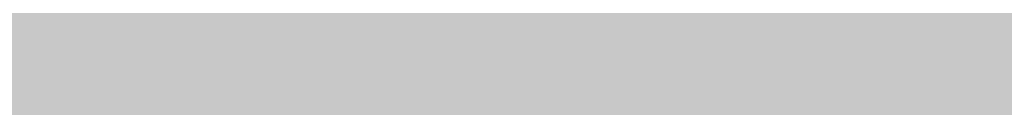
# Model space of a CAD drawing. Units: inches. Extents: x 2091 to 2899, y 967 to 2217.
# Tile 186 of 256: x 2203.16122 to 2203.18039, y 1152.24874 to 1152.25042. Entities that reach past the tile are written whole.
import ezdxf

# ---------------------------------------------------------------- set-up
doc = ezdxf.new("R2010")
doc.units = ezdxf.units.IN
doc.layers.add('A-WALL-PATT', color=141, linetype='Continuous', lineweight=13, true_color=0xadddf7)

msp = doc.modelspace()

# ---------------------------------------------------------------- hatches: boundary and pattern name
at = {"layer": 'A-WALL-PATT'}
h = msp.add_hatch(color=256, dxfattribs=at)
h.dxf.hatch_style = 1
h.paths.add_polyline_path([(2803.143603, 2050.919059), (2203.143603, 2050.919059), (2203.143603, 1090.919059), (2803.143603, 1090.919059)])
h.paths.add_polyline_path([(2635.79885, 1147.540465), (2674.524052, 1147.540465, 0.376086), (2678.529665, 1152.880202), (2678.529665, 1159.556473, 0.333335), (2674.524319, 1163.561846), (2674.524319, 1163.56185), (2674.524319, 1192.93439), (2635.805971, 1192.93439), (2597.087622, 1192.93439), (2597.087622, 1163.561846, 0.333335), (2593.082276, 1159.556473), (2593.082276, 1152.880202, 0.376086), (2597.087889, 1147.540465)], flags=0)
h.paths.add_polyline_path([(2436.010433, 1278.240778, 0.000483), (2435.952643, 1278.215027, -0.001328), (2435.935625, 1278.111693, -0.001711), (2436.11644, 1278.040758, 0.002185)], flags=0)
h.paths.add_polyline_path([(2794.143603, 1143.419059), (2794.143603, 1347.419059), (2543.370171, 1347.419059), (2543.370171, 1351.919059), (2794.143603, 1351.919059), (2794.143603, 1392.713555), (2793.947398, 1392.713555), (2793.947398, 1473.5369), (2794.143603, 1473.5369), (2794.143603, 1531.919059), (2650.143603, 1531.919059), (2650.143603, 1536.419059), (2794.143603, 1536.419059), (2794.143603, 1692.419059), (2609.375609, 1692.419059), (2609.375609, 1644.419059), (2604.875609, 1644.419059), (2604.875609, 1744.919059), (2609.375609, 1744.919059), (2609.375609, 1696.919059), (2794.143603, 1696.919059), (2794.143603, 1780.919059), (2609.643603, 1780.919059), (2493.875609, 1780.919059), (2493.875609, 1785.419059), (2609.643603, 1785.419059), (2794.143603, 1785.419059), (2794.143603, 1847.938821), (2793.951222, 1847.938821), (2793.951222, 1928.762166), (2794.143603, 1928.762166), (2794.143603, 1941.419059), (2614.143603, 1941.419059), (2614.143603, 1821.419059), (2609.643603, 1821.419059), (2609.643603, 1941.419059), (2392.143603, 1941.419059), (2392.143603, 1819.919059), (2387.643603, 1819.919059), (2387.643603, 1941.419059), (2212.143603, 1941.419059), (2212.143603, 1783.919059), (2392.143603, 1783.919059), (2392.143603, 1780.919059), (2212.143603, 1780.919059), (2212.143603, 1629.419059), (2387.643603, 1629.419059), (2387.643603, 1744.919059), (2392.143603, 1744.919059), (2392.143603, 1627.919059), (2317.143603, 1627.919059), (2317.143603, 1551.419059), (2317.143603, 1536.419059), (2459.383591, 1536.419059), (2459.383591, 1602.39648), (2463.883591, 1602.39648), (2463.883591, 1531.919059), (2456.643603, 1531.919059), (2456.643603, 1529.919059), (2452.143603, 1529.919059), (2452.143603, 1531.919059), (2312.643603, 1531.919059), (2312.643603, 1551.419059), (2306.143603, 1551.419059), (2306.143603, 1555.919059), (2308.143603, 1555.919059), (2308.143603, 1551.419059), (2312.643603, 1551.419059), (2312.643603, 1627.919059), (2212.143603, 1627.919059), (2212.143603, 1555.919059), (2270.143603, 1555.919059), (2270.143603, 1551.419059), (2212.143603, 1551.419059), (2212.143603, 1351.919059), (2272.143603, 1351.919059), (2272.143603, 1347.419059), (2212.143603, 1347.419059), (2212.143603, 1275.419059), (2308.143603, 1275.419059), (2308.143603, 1351.919059), (2452.143603, 1351.919059), (2452.143603, 1493.919059), (2456.643603, 1493.919059), (2456.643603, 1347.419059), (2312.643603, 1347.419059), (2312.643603, 1270.919059), (2212.143603, 1270.919059), (2212.143603, 1099.919059), (2281.237523, 1099.919059), (2282.871041, 1110.913803), (2282.008341, 1116.996603), (2278.557741, 1121.420403), (2268.205641, 1128.056203), (2272.087641, 1128.056203), (2273.812941, 1131.927003), (2279.420341, 1134.691903), (2285.027841, 1135.244903), (2287.615841, 1137.456803), (2288.047141, 1138.009803), (2289.341141, 1140.774703), (2291.066541, 1139.668703), (2292.360541, 1135.244903), (2295.379841, 1136.903803), (2296.242541, 1135.797903), (2297.105241, 1133.033003), (2300.124641, 1138.009803), (2303.143941, 1138.009803), (2304.437941, 1135.797903), (2303.143941, 1133.586003), (2306.594641, 1134.691903), (2307.888741, 1133.033003), (2310.908041, 1135.244903), (2313.927441, 1134.138903), (2315.62686, 1132.427102), (2308.320041, 1117.549603), (2290.203841, 1109.807903), (2288.909841, 1103.172103), (2289.272309, 1099.919059), (2434.918227, 1099.919059), (2431.593227, 1124.788059), (2429.930227, 1169.553059), (2430.927185, 1240.519694), (2435.658926, 1238.186126), (2437.135227, 1196.554059), (2438.798227, 1143.973059), (2442.678227, 1111.998059), (2446.558227, 1099.919059), (2794.143603, 1099.919059), (2794.143603, 1138.919059), (2548.032447, 1138.919059), (2548.032447, 1143.419059), (2548.032447, 1148.819059), (2546.668457, 1148.031559), (2528.685692, 1179.178622, 0.256256), (2512.032447, 1148.819059), (2512.032447, 1143.419059), (2512.032447, 1138.919059), (2507.532447, 1138.919059), (2507.532447, 1143.419059), (2507.532447, 1148.819059, 0.256256), (2490.879202, 1179.178622), (2472.896437, 1148.031559), (2471.532447, 1148.819059), (2471.532447, 1143.419059), (2467.032447, 1143.419059), (2467.032447, 1269.945786, 0.039061), (2460.909987, 1273.580059), (2467.032447, 1273.580059), (2467.032447, 1286.325364, 0.014511), (2465.216194, 1286.761905), (2467.032447, 1287.052576), (2467.032447, 1323.419059), (2471.532447, 1323.419059), (2471.532447, 1148.819059), (2489.532447, 1179.995973), (2490.896437, 1179.208473), (2490.879202, 1179.178622, -0.256256), (2507.532447, 1148.819059), (2507.532447, 1143.419059), (2512.032447, 1143.419059), (2512.032447, 1148.819059, -0.256256), (2528.685692, 1179.178622), (2528.668457, 1179.208473), (2530.032447, 1179.995973), (2548.032447, 1148.819059), (2548.032447, 1143.419059)], flags=16)
h.paths.add_polyline_path([(2607.768546, 1200.945083), (2607.768546, 1265.030625), (2597.087622, 1281.052011), (2619.784585, 1281.052011), (2627.795278, 1337.12686), (2635.79885, 1337.12686), (2643.816663, 1337.12686), (2651.827356, 1281.052011), (2674.524319, 1281.052011), (2663.843395, 1265.030625), (2663.843395, 1200.945083), (2635.805971, 1200.945083)], flags=0)
edge = h.paths.add_edge_path(flags=0)
edge.add_ellipse((13303.896215, 1272.998725), major_axis=(-10595.31304, 0.000001), ratio=0.842303870086, start_angle=0.6282372191, end_angle=0.6465540999, ccw=False)
edge.add_ellipse((2711.70045, 1156.852678), major_axis=(2.219769, 0), ratio=0.84230387, start_angle=111.535244, end_angle=180.628237, ccw=False)
edge.add_ellipse((13303.156292, 1272.998725), major_axis=(-10593.026306, 0), ratio=0.842303869544, start_angle=0.5282714718, end_angle=0.6465540971, ccw=False)
edge.add_line((2710.764596, 1175.333295), (2710.129986, 1175.333295))
edge.add_ellipse((2710.129986, 1176.579775), major_axis=(1.479846, 0), ratio=0.84230387, start_angle=180, end_angle=270, ccw=False)
edge.add_line((2708.65014, 1176.579775), (2708.65014, 1200.782914))
edge.add_ellipse((2710.129986, 1200.782914), major_axis=(1.479846, 0), ratio=0.84230387, start_angle=90, end_angle=180, ccw=False)
edge.add_line((2710.129986, 1202.029394), (2710.465075, 1202.029394))
edge.add_ellipse((13303.156292, 1272.998725), major_axis=(-10593.026306, 0), ratio=0.842303869544, start_angle=-0.0902290886, end_angle=0.3838667788, ccw=False)
edge.add_ellipse((2710.129986, 1290.927031), major_axis=(-1.479846, 0), ratio=0.84230387, start_angle=0, end_angle=90, ccw=False)
edge.add_line((2708.65014, 1290.927031), (2708.65014, 1315.13017))
edge.add_ellipse((2710.129986, 1315.13017), major_axis=(-1.479846, 0), ratio=0.84230387, start_angle=-90, end_angle=0, ccw=False)
edge.add_line((2710.129986, 1316.37665), (2710.706314, 1316.37665))
edge.add_ellipse((3238.40172, 1296.289566), major_axis=(528.234, 0), ratio=0.8423038695, start_angle=176.34957241, end_angle=177.82004969, ccw=False)
edge.add_ellipse((2775.063043, 1071.450696), major_axis=(313.307761, 0), ratio=0.8423038695, start_angle=102.12596555, end_angle=103.78052899, ccw=False)
edge.add_ellipse((2775.063043, 1078.305698), major_axis=(-305.302891, 0), ratio=0.8423038695, start_angle=-79.790461, end_angle=-77.55537271, ccw=False)
edge.add_ellipse((2695.141767, 1541.975383), major_axis=(-250.960216, 0), ratio=0.8423038695, start_angle=99.25656601, end_angle=102.55493264)
edge.add_line((2741.410326, 1334.214255), (2747.132545, 1337.378477))
edge.add_ellipse((2747.538616, 1336.857478), major_axis=(-0.739923, 0), ratio=0.8423039, start_angle=270, end_angle=307.93313, ccw=False)
edge.add_ellipse((2747.538616, 1336.857478), major_axis=(-0.739923, 0), ratio=0.8423039, start_angle=232.06687, end_angle=270, ccw=False)
edge.add_line((2747.944687, 1337.378477), (2753.666906, 1334.214255))
edge.add_ellipse((2799.935466, 1541.975383), major_axis=(250.960216, 0), ratio=0.8423038695, start_angle=257.44506736, end_angle=260.74343399)
edge.add_ellipse((2720.014189, 1078.305698), major_axis=(305.302891, 0), ratio=0.8423038695, start_angle=77.55537271, end_angle=79.790461, ccw=False)
edge.add_ellipse((2720.014189, 1071.450696), major_axis=(-313.307761, 0), ratio=0.8423038695, start_angle=256.21947101, end_angle=257.87403445, ccw=False)
edge.add_ellipse((2256.675512, 1296.289566), major_axis=(-528.234, 0), ratio=0.8423038695, start_angle=182.17995031, end_angle=183.65042759, ccw=False)
edge.add_line((2784.370918, 1316.37665), (2784.947247, 1316.37665))
edge.add_ellipse((2784.947247, 1315.13017), major_axis=(1.479846, 0), ratio=0.84230387, start_angle=0, end_angle=90, ccw=False)
edge.add_line((2786.427093, 1315.13017), (2786.427093, 1290.927031))
edge.add_ellipse((2784.947247, 1290.927031), major_axis=(1.479846, 0), ratio=0.84230387, start_angle=270, end_angle=360, ccw=False)
edge.add_ellipse((-7808.07906, 1272.998725), major_axis=(10593.026306, 0), ratio=0.842303869544, start_angle=-0.3838667788, end_angle=0.0902290886, ccw=False)
edge.add_line((2784.612157, 1202.029394), (2784.947247, 1202.029394))
edge.add_ellipse((2784.947247, 1200.782914), major_axis=(1.479846, 0), ratio=0.84230387, start_angle=0, end_angle=90, ccw=False)
edge.add_line((2786.427093, 1200.782914), (2786.427093, 1176.579775))
edge.add_ellipse((2784.947247, 1176.579775), major_axis=(-1.479846, 0), ratio=0.84230387, start_angle=90, end_angle=180, ccw=False)
edge.add_line((2784.947247, 1175.333295), (2784.312636, 1175.333295))
edge.add_ellipse((-7808.07906, 1272.998725), major_axis=(10593.026306, 0), ratio=0.842303869544, start_angle=-0.6186431963, end_angle=-0.5282714718, ccw=False)
edge.add_ellipse((2783.376783, 1156.852678), major_axis=(-2.219769, 0), ratio=0.84230387, start_angle=179.371763, end_angle=248.464757, ccw=False)
edge.add_ellipse((-7808.818983, 1272.998725), major_axis=(-10595.31304, 0.000004), ratio=0.842303865762, start_angle=179.3534459226, end_angle=179.3717628034, ccw=False)
edge.add_ellipse((2780.297303, 1153.500793), major_axis=(-5.246426, 0), ratio=0.84230387, start_angle=90, end_angle=179.353446, ccw=False)
edge.add_line((2780.297303, 1149.081708), (2714.77993, 1149.081708))
edge.add_ellipse((2714.77993, 1153.500793), major_axis=(5.246426, 0), ratio=0.84230387, start_angle=180.646554, end_angle=270, ccw=False)
edge = h.paths.add_edge_path(flags=0)
edge.add_line((2718.187367, 1151.007833), (2718.187367, 1170.472364))
edge.add_ellipse((2721.14706, 1170.472364), major_axis=(-2.959692, 0), ratio=0.84230387, start_angle=-90, end_angle=0, ccw=False)
edge.add_line((2721.14706, 1172.965324), (2773.930173, 1172.965324))
edge.add_ellipse((2773.930173, 1170.472364), major_axis=(-2.959692, 0), ratio=0.84230387, start_angle=180, end_angle=270, ccw=False)
edge.add_line((2776.889865, 1170.472364), (2776.889865, 1151.007833))
edge.add_line((2776.889865, 1151.007833), (2718.187367, 1151.007833))
edge = h.paths.add_edge_path(flags=0)
edge.add_line((2718.187367, 1180.23415), (2718.187367, 1199.057834))
edge.add_ellipse((2747.538616, 1320.39864), major_axis=(147.017924, 0), ratio=0.8423038695, start_angle=256.40186531, end_angle=283.59813469)
edge.add_line((2776.889865, 1199.057834), (2776.889865, 1180.23415))
edge.add_ellipse((2747.538616, 1301.574956), major_axis=(147.017924, 0), ratio=0.8423038695, start_angle=256.40186531, end_angle=283.59813469, ccw=False)
edge = h.paths.add_edge_path(flags=0)
edge.add_ellipse((13303.156292, 1272.998725), major_axis=(-10591.54646, 0), ratio=0.842303869555, start_angle=0.0555943135, end_angle=0.3777641939, ccw=False)
edge.add_line((2711.616859, 1262.72171), (2715.667408, 1249.495396))
edge.add_ellipse((6413.891963, 1241.691919), major_axis=(-3698.236159, 0), ratio=0.84230386955, start_angle=-0.120897369, end_angle=0.364076349)
edge.add_line((2715.761038, 1218.192455), (2711.934307, 1203.167361))
edge = h.paths.add_edge_path(flags=0)
edge.add_line((2718.187367, 1251.074566), (2716.002485, 1267.450435))
edge.add_ellipse((2742.151175, 1202.18954), major_axis=(81.772585, 0), ratio=0.84230387, start_angle=94.27742096, end_angle=111.8349538, ccw=False)
edge.add_line((2737.009748, 1270.930626), (2758.067484, 1270.930626))
edge.add_ellipse((2752.926058, 1202.18954), major_axis=(81.772585, 0), ratio=0.84230387, start_angle=68.1650462, end_angle=85.72257904, ccw=False)
edge.add_line((2779.074747, 1267.450435), (2776.889865, 1251.074566))
edge.add_ellipse((2750.338059, 1187.885356), major_axis=(79.579664, 0), ratio=0.84230387, start_angle=67.20808512, end_angle=85.1299304)
edge.add_line((2756.034656, 1254.743656), (2739.042576, 1254.743656))
edge.add_ellipse((2744.739174, 1187.885356), major_axis=(79.579664, 0), ratio=0.84230387, start_angle=94.8700696, end_angle=112.79191488)
edge = h.paths.add_edge_path(flags=0)
edge.add_line((2783.142926, 1203.167361), (2779.316194, 1218.192455))
edge.add_ellipse((-918.81473, 1241.691919), major_axis=(3698.236159, 0), ratio=0.84230386955, start_angle=-0.364076349, end_angle=0.120897369)
edge.add_line((2779.409825, 1249.495396), (2783.460373, 1262.72171))
edge.add_ellipse((-7808.07906, 1272.998725), major_axis=(-10591.54646, 0), ratio=0.84230386954, start_angle=179.6222358061, end_angle=179.9444056865, ccw=False)
edge = h.paths.add_edge_path(flags=0)
edge.add_ellipse((2734.200892, 1286.69044), major_axis=(-0.356609, 6.340078), ratio=0.60383358, start_angle=89.0020143, end_angle=253.657408, ccw=False)
edge.add_line((2730.369001, 1286.541806), (2730.369001, 1301.35198))
edge.add_line((2730.369001, 1301.35198), (2735.913311, 1305.214803))
edge.add_ellipse((2736.384917, 1304.734561), major_axis=(0.739923, 0), ratio=0.8423039, start_angle=90, end_angle=134.480211, ccw=False)
edge.add_line((2736.384917, 1305.357801), (2738.032783, 1305.357801))
edge.add_line((2738.032783, 1305.357801), (2738.032783, 1307.707927))
edge.add_ellipse((2794.201642, 1307.707927), major_axis=(56.168859, 0), ratio=0.84230387, start_angle=150.5614304, end_angle=180, ccw=False)
edge.add_ellipse((2700.875591, 1307.707927), major_axis=(-56.168859, 0), ratio=0.84230387, start_angle=180, end_angle=209.4385696, ccw=False)
edge.add_line((2757.04445, 1307.707927), (2757.04445, 1305.357801))
edge.add_line((2757.04445, 1305.357801), (2758.692316, 1305.357801))
edge.add_ellipse((2758.692316, 1304.734561), major_axis=(-0.739923, 0), ratio=0.8423039, start_angle=225.519789, end_angle=270, ccw=False)
edge.add_line((2759.163922, 1305.214803), (2764.708231, 1301.35198))
edge.add_line((2764.708231, 1301.35198), (2764.708231, 1286.541806))
edge.add_ellipse((2760.87634, 1286.69044), major_axis=(0.356609, 6.340078), ratio=0.60383358, start_angle=106.342592, end_angle=270.9979857, ccw=False)
edge.add_line((2757.04445, 1285.79709), (2757.04445, 1307.707927))
edge.add_ellipse((2700.875591, 1307.707927), major_axis=(-56.168859, 0), ratio=0.84230387, start_angle=180, end_angle=209.4385696)
edge.add_ellipse((2794.201642, 1307.707927), major_axis=(56.168859, 0), ratio=0.84230387, start_angle=150.5614304, end_angle=180)
edge.add_line((2738.032783, 1307.707927), (2738.032783, 1285.79709))
h.paths.add_polyline_path([(2417.812273, 1104.449704), (2413.492273, 1102.529704), (2410.612273, 1103.969704), (2409.172273, 1106.369704), (2407.252273, 1107.329704), (2406.292273, 1109.729704), (2405.332273, 1114.049704), (2405.332273, 1117.889704), (2406.292273, 1120.129704), (2407.252273, 1119.809704), (2408.848322, 1118.327658), (2410.173945, 1119.42417), (2410.211273, 1120.405704), (2411.040731, 1121.419054), (2410.699273, 1119.858704), (2410.173945, 1119.42417), (2410.088452, 1117.176109), (2411.132836, 1116.206324), (2413.972273, 1119.329704), (2416.852273, 1120.769704), (2416.869721, 1120.798784), (2417.035071, 1119.405116), (2417.896213, 1118.143384), (2418.292273, 1118.369704), (2419.544447, 1120.039269), (2419.360915, 1118.387487), (2419.032108, 1119.356151), (2418.398939, 1118.511926), (2419.252273, 1114.529704), (2418.794091, 1107.198795)], flags=0)
h.paths.add_polyline_path([(2508.870171, 1347.419059), (2508.370171, 1347.419059), (2508.370171, 1351.919059), (2508.870171, 1351.919059)], flags=0)
h.paths.add_polyline_path([(2473.370171, 1347.419059), (2472.370171, 1347.419059), (2467.870171, 1347.419059), (2467.870171, 1455.419059), (2472.370171, 1455.419059), (2472.370171, 1352.419059), (2473.370171, 1352.419059)], flags=0)
h.paths.add_polyline_path([(2352.106244, 1217.446197), (2349.226244, 1218.886197), (2347.786244, 1221.286197), (2345.866244, 1222.246197), (2344.906244, 1224.646197), (2343.946244, 1228.966197), (2343.946244, 1232.806197), (2344.906244, 1235.046197), (2345.866244, 1234.726197), (2347.462293, 1233.244152), (2348.787916, 1234.340663), (2348.825244, 1235.322197), (2349.654702, 1236.335547), (2349.313244, 1234.775197), (2348.787916, 1234.340663), (2348.702423, 1232.092603), (2349.746807, 1231.122817), (2352.586244, 1234.246197), (2355.466244, 1235.686197), (2355.483692, 1235.715277), (2355.649043, 1234.321609), (2356.510185, 1233.059877), (2356.906244, 1233.286197), (2358.158418, 1234.955762), (2357.974887, 1233.30398), (2357.646079, 1234.272644), (2357.012911, 1233.428419), (2357.866244, 1229.446197), (2357.408062, 1222.115288), (2356.426244, 1219.366197)], flags=0)
h.paths.add_polyline_path([(2348.2968, 1112.22442), (2347.0138, 1112.31042), (2345.5298, 1114.12742), (2345.7318, 1115.85842), (2346.8118, 1116.98242), (2346.8118, 1114.64642), (2345.8668, 1114.21442), (2346.8798, 1114.30042)], flags=0)
h.paths.add_polyline_path([(2347.0138, 1110.92642), (2346.2718, 1110.49342), (2346.6098, 1111.18642)], flags=0)
h.paths.add_polyline_path([(2345.8668, 1118.19442), (2345.5298, 1117.32942), (2343.7078, 1118.02142), (2344.3828, 1118.62642)], flags=0)
h.paths.add_polyline_path([(2346.6768, 1109.28242), (2346.0698, 1108.07142), (2345.8668, 1110.06142)], flags=0)
h.paths.add_polyline_path([(2345.0568, 1119.75142), (2343.6398, 1119.75142), (2343.9778, 1121.13542)], flags=0)
h.paths.add_polyline_path([(2345.2598, 1116.55042), (2345.1248, 1115.85842), (2344.9218, 1115.68542), (2344.7198, 1116.37742)], flags=0)
h.paths.add_polyline_path([(2345.6648, 1112.31042), (2345.4618, 1111.53242), (2344.0448, 1111.96442), (2344.6518, 1112.57042)], flags=0)
h.paths.add_polyline_path([(2345.1918, 1113.34942), (2344.4498, 1113.86842), (2344.7198, 1114.38742)], flags=0)
h.paths.add_polyline_path([(2344.6518, 1116.80942), (2344.1798, 1115.68542), (2344.6518, 1115.33942), (2343.9098, 1114.90642), (2343.0328, 1115.94442), (2343.6398, 1116.46342)], flags=0)
h.paths.add_polyline_path([(2345.8668, 1106.68642), (2344.9898, 1105.56242), (2344.5168, 1106.60042)], flags=0)
h.paths.add_polyline_path([(2344.8548, 1110.06142), (2344.5168, 1109.28242), (2344.1128, 1109.71542)], flags=0)
h.paths.add_polyline_path([(2344.0448, 1113.52242), (2343.4378, 1113.08942), (2342.7628, 1113.95442)], flags=0)
h.paths.add_polyline_path([(2344.3148, 1111.01242), (2342.9648, 1110.32042), (2342.9648, 1111.09942)], flags=0)
h.paths.add_polyline_path([(2345.1248, 1104.69742), (2344.5848, 1103.74542), (2344.4498, 1104.26442)], flags=0)
h.paths.add_polyline_path([(2342.8298, 1121.22242), (2341.7498, 1120.53042), (2340.5358, 1121.04942), (2340.1308, 1121.82842), (2340.6708, 1122.95242), (2341.1428, 1121.82842), (2341.6148, 1122.00142)], flags=0)
h.paths.add_polyline_path([(2342.9648, 1119.75142), (2343.0328, 1118.45342), (2342.0878, 1118.02142), (2342.0198, 1119.49142)], flags=0)
h.paths.add_polyline_path([(2342.6948, 1116.89642), (2341.9528, 1116.63642), (2342.0198, 1117.32942)], flags=0)
h.paths.add_polyline_path([(2343.0328, 1112.22442), (2342.0198, 1111.79142), (2341.5478, 1112.22442), (2342.3578, 1113.34942)], flags=0)
h.paths.add_polyline_path([(2343.7748, 1104.43742), (2342.6278, 1102.88042), (2342.6948, 1104.61042), (2343.4378, 1105.12942)], flags=0)
h.paths.add_polyline_path([(2342.0198, 1115.07942), (2340.8058, 1115.51242), (2340.9408, 1116.37742)], flags=0)
h.paths.add_polyline_path([(2341.4808, 1120.09742), (2341.4808, 1119.40542), (2341.0758, 1119.57842), (2341.1428, 1120.09742)], flags=0)
h.paths.add_polyline_path([(2341.8178, 1114.47342), (2340.9408, 1113.08942), (2340.8058, 1114.56042)], flags=0)
h.paths.add_polyline_path([(2341.1428, 1118.54042), (2340.9408, 1116.98242), (2339.0508, 1117.67542), (2339.0508, 1118.62642)], flags=0)
h.paths.add_polyline_path([(2342.6948, 1101.66842), (2341.9528, 1101.84142), (2342.5598, 1102.36142)], flags=0)
h.paths.add_polyline_path([(2340.3328, 1119.66542), (2338.4438, 1119.57842), (2337.9038, 1120.35742), (2339.6578, 1120.61642)], flags=0)
h.paths.add_polyline_path([(2340.3328, 1115.33942), (2340.0628, 1113.69542), (2339.3878, 1115.33942)], flags=0)
h.paths.add_polyline_path([(2341.8178, 1103.83142), (2341.5478, 1102.88042), (2341.1428, 1103.65842)], flags=0)
h.paths.add_polyline_path([(2339.0508, 1122.86642), (2337.2958, 1121.82842), (2337.0938, 1123.12542), (2337.7688, 1123.81842)], flags=0)
h.paths.add_polyline_path([(2339.1178, 1121.74142), (2338.8478, 1121.22242), (2338.1738, 1121.04942), (2338.3758, 1121.56842)], flags=0)
h.paths.add_polyline_path([(2339.1858, 1119.31942), (2338.6458, 1118.71342), (2338.2408, 1118.10742), (2338.2408, 1118.88642)], flags=0)
h.paths.add_polyline_path([(2341.1428, 1101.92842), (2340.6028, 1101.23642), (2340.0628, 1101.84142), (2340.6028, 1102.36142)], flags=0)
h.paths.add_polyline_path([(2337.6338, 1117.76142), (2336.6208, 1118.28042), (2337.2958, 1118.97242)], flags=0)
h.paths.add_polyline_path([(2336.8238, 1119.57842), (2334.7988, 1118.97242), (2335.2038, 1120.35742), (2336.5538, 1120.87642)], flags=0)
h.paths.add_polyline_path([(2339.1178, 1100.45742), (2337.3638, 1100.54342), (2336.7558, 1101.23642)], flags=0)
h.paths.add_polyline_path([(2336.3508, 1122.43342), (2336.0138, 1121.91442), (2334.9338, 1122.43342), (2334.5288, 1123.47142), (2335.7438, 1122.77942)], flags=0)
h.paths.add_polyline_path([(2334.7318, 1120.87642), (2334.2588, 1120.35742), (2334.0568, 1120.78942), (2334.5968, 1121.30842)], flags=0)
h.paths.add_polyline_path([(2334.4618, 1122.17442), (2332.5718, 1121.30842), (2331.3568, 1122.17442), (2332.0998, 1122.86642)], flags=0)
h.paths.add_polyline_path([(2334.2588, 1118.54042), (2333.3818, 1118.45342), (2333.6518, 1119.31942)], flags=0)
h.paths.add_polyline_path([(2335.5418, 1102.27442), (2334.1918, 1102.62042), (2335.2718, 1103.31242)], flags=0)
h.paths.add_polyline_path([(2332.7068, 1119.66542), (2331.6948, 1120.44342), (2332.5048, 1120.78942)], flags=0)
h.paths.add_polyline_path([(2334.7318, 1101.14942), (2333.5168, 1101.58242), (2333.9888, 1101.75542)], flags=0)
h.paths.add_polyline_path([(2332.6398, 1116.63642), (2331.0868, 1116.29042), (2331.9648, 1118.19442)], flags=0)
h.paths.add_polyline_path([(2330.7498, 1121.56842), (2330.2768, 1120.27042), (2328.5228, 1119.31942), (2328.9948, 1121.04942)], flags=0)
h.paths.add_polyline_path([(2330.7498, 1118.62642), (2330.0078, 1117.50242), (2329.8728, 1118.02142)], flags=0)
h.paths.add_polyline_path([(2332.0998, 1102.36142), (2330.5468, 1102.01442), (2331.6948, 1102.96642)], flags=0)
h.paths.add_polyline_path([(2329.5348, 1113.60842), (2329.0628, 1112.31042), (2328.5898, 1113.34942)], flags=0)
h.paths.add_polyline_path([(2328.3878, 1117.84842), (2327.5098, 1116.55042), (2327.1728, 1117.76142)], flags=0)
h.paths.add_polyline_path([(2329.7378, 1106.51342), (2329.5348, 1105.30242), (2328.2528, 1106.08142)], flags=0)
h.paths.add_polyline_path([(2328.6578, 1114.38742), (2328.0498, 1114.12742), (2328.3198, 1114.90642)], flags=0)
h.paths.add_polyline_path([(2328.3198, 1112.22442), (2327.1058, 1112.13742), (2326.7008, 1112.65642)], flags=0)
h.paths.add_polyline_path([(2326.9028, 1115.25242), (2326.7008, 1114.12742), (2325.2158, 1113.60842), (2326.0928, 1115.33942)], flags=0)
h.paths.add_polyline_path([(2326.6328, 1108.33042), (2326.0928, 1107.37942), (2325.8908, 1108.50342), (2326.4978, 1109.10942)], flags=0)
h.paths.add_polyline_path([(2615.143603, 1531.919059), (2609.643603, 1531.919059), (2609.643603, 1620.419059), (2614.143603, 1620.419059), (2614.143603, 1536.419059), (2615.143603, 1536.419059)], flags=0)
h.paths.add_polyline_path([(2545.143603, 1563.419059), (2464.143603, 1563.419059), (2464.143603, 1632.419059), (2509.143603, 1632.419059), (2509.143603, 1627.919059), (2509.143603, 1603.919059), (2468.643603, 1603.919059), (2468.643603, 1567.919059), (2540.643603, 1567.919059), (2540.643603, 1591.919059), (2545.143603, 1591.919059)], flags=0)
h.paths.add_polyline_path([(2388.969048, 1549.985735), (2357.434181, 1549.985735), (2357.434181, 1623.360778), (2399.362777, 1623.360778), (2435.689465, 1623.360778), (2435.592547, 1602.559273), (2435.592547, 1602.39648), (2388.969048, 1602.39648)], flags=0)
h.paths.add_polyline_path([(2388.880628, 1555.809151), (2374.904429, 1555.809151), (2374.904429, 1600.571564), (2374.904429, 1615.457645), (2406.350877, 1615.457645), (2406.350877, 1618.939431), (2412.174293, 1615.457645), (2406.350877, 1611.97586), (2406.350877, 1615.457645), (2388.880628, 1615.457645)], flags=0)
h.paths.add_polyline_path([(2568.875609, 1644.419059), (2453.375609, 1644.419059), (2453.375609, 1785.419059), (2457.875609, 1785.419059), (2457.875609, 1648.919059), (2568.875609, 1648.919059)], flags=0)
h.paths.add_polyline_path([(2212.143603, 1945.919059), (2212.143603, 2041.919059), (2794.143603, 2041.919059), (2794.143603, 1945.919059)], flags=16)
h.paths.add_polyline_path([(2271.082728, 1964.317238), (2776.852968, 1964.317238), (2776.852968, 2037.169623), (2271.082728, 2037.169623)], flags=8)
h.paths.add_polyline_path([(2380.649285, 1536.824144), (2461.040809, 1536.824144), (2461.040809, 1554.652587), (2380.649285, 1554.652587)], flags=8)
h.paths.add_polyline_path([(2240.755709, 1609.725451), (2309.185829, 1609.725451), (2309.185829, 1617.698204), (2240.755709, 1617.698204)], flags=8)
h.paths.add_polyline_path([(2212.677255, 1313.504102), (2282.59152, 1313.504102), (2282.59152, 1322.745239), (2212.677255, 1322.745239)], flags=8)
h.paths.add_polyline_path([(2457.111976, 1114.778574), (2558.481581, 1114.778574), (2558.481581, 1142.219682), (2457.111976, 1142.219682)], flags=8)
h.paths.add_polyline_path([(2473.442337, 1273.010067), (2604.641226, 1273.010067), (2604.641226, 1318.346935), (2473.442337, 1318.346935)], flags=8)
h.paths.add_polyline_path([(2638.876302, 1626.977432), (2684.250367, 1627.976738), (2684.038483, 1637.597494), (2638.664417, 1636.598188)], flags=8)
h.paths.add_polyline_path([(2537.590554, 1453.793447), (2628.389547, 1453.793447), (2628.389547, 1475.344811), (2537.590554, 1475.344811)], flags=8)
h.paths.add_polyline_path([(2504.137638, 1714.632397), (2554.647187, 1714.632397), (2554.647187, 1730.237712), (2504.137638, 1730.237712)], flags=8)
h.paths.add_polyline_path([(2487.501181, 1575.651872), (2535.097121, 1575.651872), (2535.097121, 1598.377646), (2487.501181, 1598.377646)], flags=8)
h.paths.add_polyline_path([(2709.0994, 1735.710278), (2740.016601, 1735.710278), (2740.016601, 1749.937641), (2709.0994, 1749.937641)], flags=8)
h.paths.add_polyline_path([(2442.438424, 1792.171657), (2564.728835, 1792.171657), (2564.728835, 1842.000163), (2442.438424, 1842.000163)], flags=8)
h.paths.add_polyline_path([(2655.815801, 1809.644076), (2789.520142, 1806.693796), (2790.084977, 1832.291638), (2656.380635, 1835.241918)], flags=8)
h.paths.add_polyline_path([(2234.842697, 1797.720143), (2368.592851, 1794.768852), (2369.160718, 1820.504132), (2235.410564, 1823.455423)], flags=8)
h.paths.add_polyline_path([(2245.138466, 1644.006335), (2398.427733, 1640.6239), (2398.994842, 1666.32482), (2245.705575, 1669.707255)], flags=8)
h.paths.add_polyline_path([(2306.142847, 1431.168519), (2413.768314, 1428.793687), (2414.333148, 1454.391529), (2306.707682, 1456.76636)], flags=8)
h.paths.add_polyline_path([(2306.834582, 1458.233145), (2393.380484, 1456.323449), (2393.932808, 1481.354358), (2307.386907, 1483.264054)], flags=8)

doc.saveas('drawing.dxf')
